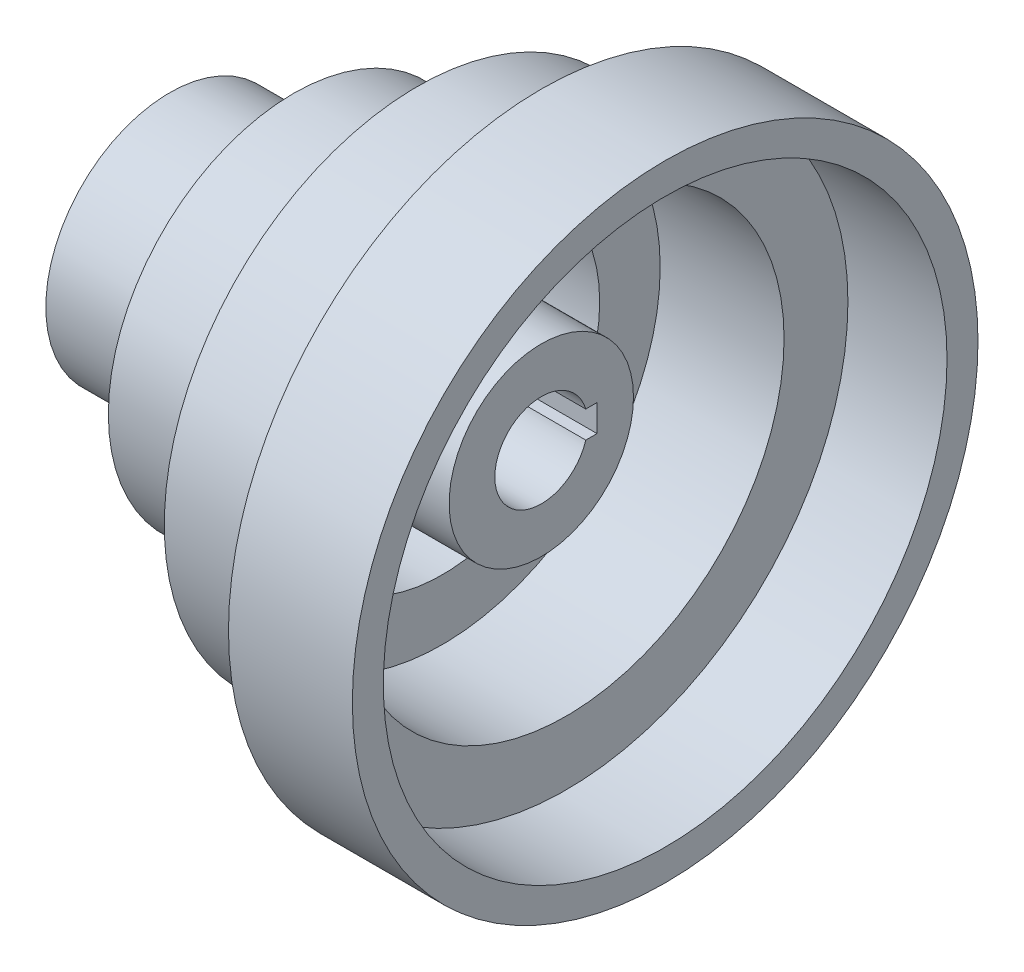
ISO-10303-21;
HEADER;
FILE_DESCRIPTION(('STEP AP214'),'2;1');
FILE_NAME('part.step','',(''),(''),'','','');
FILE_SCHEMA(('AUTOMOTIVE_DESIGN { 1 0 10303 214 1 1 1 1 }'));
ENDSEC;
DATA;
#1=APPLICATION_CONTEXT('core data for automotive mechanical design processes');
#2=APPLICATION_PROTOCOL_DEFINITION('international standard','automotive_design',2000,#1);
#3=PRODUCT_CONTEXT('',#1,'mechanical');
#4=PRODUCT('Part','Part','',(#3));
#5=PRODUCT_RELATED_PRODUCT_CATEGORY('part','',(#4));
#6=PRODUCT_DEFINITION_FORMATION('','',#4);
#7=PRODUCT_DEFINITION_CONTEXT('part definition',#1,'design');
#8=PRODUCT_DEFINITION('design','',#6,#7);
#9=PRODUCT_DEFINITION_SHAPE('','',#8);
#10=(LENGTH_UNIT() NAMED_UNIT(*) SI_UNIT(.MILLI.,.METRE.));
#11=(NAMED_UNIT(*) PLANE_ANGLE_UNIT() SI_UNIT($,.RADIAN.));
#12=(NAMED_UNIT(*) SI_UNIT($,.STERADIAN.) SOLID_ANGLE_UNIT());
#13=UNCERTAINTY_MEASURE_WITH_UNIT(LENGTH_MEASURE(1.E-05),#10,'distance_accuracy_value','');
#14=(GEOMETRIC_REPRESENTATION_CONTEXT(3) GLOBAL_UNCERTAINTY_ASSIGNED_CONTEXT((#13)) GLOBAL_UNIT_ASSIGNED_CONTEXT((#10,
#11,#12)) REPRESENTATION_CONTEXT('',''));
#15=CARTESIAN_POINT('',(0.,0.,0.));
#16=DIRECTION('',(0.,0.,1.));
#17=DIRECTION('',(1.,0.,0.));
#18=AXIS2_PLACEMENT_3D('',#15,#16,#17);
#19=CARTESIAN_POINT('',(151.689826596154,0.,0.));
#20=DIRECTION('',(1.,0.,0.));
#21=DIRECTION('',(0.,0.,-1.));
#22=AXIS2_PLACEMENT_3D('',#19,#20,#21);
#23=CYLINDRICAL_SURFACE('',#22,15.);
#24=DIRECTION('',(1.,0.,0.));
#25=VECTOR('',#24,1.);
#26=CARTESIAN_POINT('',(151.689826596154,4.34007504449317,-14.3584034143134));
#27=LINE('',#26,#25);
#28=CARTESIAN_POINT('',(64.9299911946379,4.34007504449317,-14.3584034143134));
#29=VERTEX_POINT('',#28);
#30=CARTESIAN_POINT('',(-55.0700088053621,4.34007504449317,-14.3584034143134));
#31=VERTEX_POINT('',#30);
#32=EDGE_CURVE('E58',#29,#31,#27,.F.);
#33=ORIENTED_EDGE('',*,*,#32,.F.);
#34=CARTESIAN_POINT('',(64.9299911946379,0.,0.));
#35=DIRECTION('',(1.,0.,0.));
#36=DIRECTION('',(0.,0.,-1.));
#37=AXIS2_PLACEMENT_3D('',#34,#35,#36);
#38=CIRCLE('',#37,15.);
#39=CARTESIAN_POINT('',(64.9299911946379,-4.34007504449317,-14.3584034143134));
#40=VERTEX_POINT('',#39);
#41=EDGE_CURVE('E102',#29,#40,#38,.T.);
#42=ORIENTED_EDGE('',*,*,#41,.T.);
#43=DIRECTION('',(1.,0.,0.));
#44=VECTOR('',#43,1.);
#45=CARTESIAN_POINT('',(151.689826596154,-4.34007504449317,-14.3584034143134));
#46=LINE('',#45,#44);
#47=CARTESIAN_POINT('',(-55.0700088053621,-4.34007504449317,-14.3584034143134));
#48=VERTEX_POINT('',#47);
#49=EDGE_CURVE('E52',#48,#40,#46,.T.);
#50=ORIENTED_EDGE('',*,*,#49,.F.);
#51=CARTESIAN_POINT('',(-55.0700088053621,0.,0.));
#52=DIRECTION('',(1.,0.,0.));
#53=DIRECTION('',(0.,0.,-1.));
#54=AXIS2_PLACEMENT_3D('',#51,#52,#53);
#55=CIRCLE('',#54,15.);
#56=EDGE_CURVE('E100',#31,#48,#55,.T.);
#57=ORIENTED_EDGE('',*,*,#56,.F.);
#58=EDGE_LOOP('',(#33,#42,#50,#57));
#59=FACE_BOUND('',#58,.T.);
#60=ADVANCED_FACE('F39',(#59),#23,.F.);
#61=CARTESIAN_POINT('',(-55.0700088053621,15.,0.));
#62=DIRECTION('',(-1.,0.,0.));
#63=DIRECTION('',(0.,0.,1.));
#64=AXIS2_PLACEMENT_3D('',#61,#62,#63);
#65=PLANE('',#64);
#66=DIRECTION('',(0.,0.,-1.));
#67=VECTOR('',#66,1.);
#68=CARTESIAN_POINT('',(-55.0700088053621,4.34007504449317,0.));
#69=LINE('',#68,#67);
#70=CARTESIAN_POINT('',(-55.0700088053621,4.34007504449317,-18.));
#71=VERTEX_POINT('',#70);
#72=EDGE_CURVE('E105',#31,#71,#69,.T.);
#73=ORIENTED_EDGE('',*,*,#72,.F.);
#74=ORIENTED_EDGE('',*,*,#56,.T.);
#75=DIRECTION('',(0.,0.,1.));
#76=VECTOR('',#75,1.);
#77=CARTESIAN_POINT('',(-55.0700088053621,-4.34007504449317,0.));
#78=LINE('',#77,#76);
#79=CARTESIAN_POINT('',(-55.0700088053621,-4.34007504449317,-18.));
#80=VERTEX_POINT('',#79);
#81=EDGE_CURVE('E86',#80,#48,#78,.T.);
#82=ORIENTED_EDGE('',*,*,#81,.F.);
#83=DIRECTION('',(0.,-1.,0.));
#84=VECTOR('',#83,1.);
#85=CARTESIAN_POINT('',(-55.0700088053621,15.,-18.));
#86=LINE('',#85,#84);
#87=EDGE_CURVE('E76',#71,#80,#86,.T.);
#88=ORIENTED_EDGE('',*,*,#87,.F.);
#89=EDGE_LOOP('',(#73,#74,#82,#88));
#90=FACE_BOUND('',#89,.T.);
#91=CARTESIAN_POINT('',(-55.0700088053621,0.,0.));
#92=DIRECTION('',(1.,0.,0.));
#93=DIRECTION('',(0.,0.,-1.));
#94=AXIS2_PLACEMENT_3D('',#91,#92,#93);
#95=CIRCLE('',#94,40.);
#96=CARTESIAN_POINT('',(-55.0700088053621,0.,-40.));
#97=VERTEX_POINT('',#96);
#98=EDGE_CURVE('E155',#97,#97,#95,.T.);
#99=ORIENTED_EDGE('',*,*,#98,.F.);
#100=EDGE_LOOP('',(#99));
#101=FACE_BOUND('',#100,.T.);
#102=ADVANCED_FACE('F94',(#90,#101),#65,.T.);
#103=CARTESIAN_POINT('',(151.689826596154,0.,0.));
#104=DIRECTION('',(1.,0.,0.));
#105=DIRECTION('',(0.,0.,-1.));
#106=AXIS2_PLACEMENT_3D('',#103,#104,#105);
#107=CYLINDRICAL_SURFACE('',#106,40.);
#108=ORIENTED_EDGE('',*,*,#98,.T.);
#109=EDGE_LOOP('',(#108));
#110=FACE_BOUND('',#109,.T.);
#111=CARTESIAN_POINT('',(-15.0700088053621,0.,0.));
#112=DIRECTION('',(1.,0.,0.));
#113=DIRECTION('',(0.,0.,-1.));
#114=AXIS2_PLACEMENT_3D('',#111,#112,#113);
#115=CIRCLE('',#114,40.);
#116=CARTESIAN_POINT('',(-15.0700088053621,0.,-40.));
#117=VERTEX_POINT('',#116);
#118=EDGE_CURVE('E149',#117,#117,#115,.T.);
#119=ORIENTED_EDGE('',*,*,#118,.F.);
#120=EDGE_LOOP('',(#119));
#121=FACE_BOUND('',#120,.T.);
#122=ADVANCED_FACE('F166',(#110,#121),#107,.T.);
#123=CARTESIAN_POINT('',(-15.0700088053621,40.,0.));
#124=DIRECTION('',(-1.,0.,0.));
#125=DIRECTION('',(0.,0.,1.));
#126=AXIS2_PLACEMENT_3D('',#123,#124,#125);
#127=PLANE('',#126);
#128=ORIENTED_EDGE('',*,*,#118,.T.);
#129=EDGE_LOOP('',(#128));
#130=FACE_BOUND('',#129,.T.);
#131=CARTESIAN_POINT('',(-15.0700088053621,0.,0.));
#132=DIRECTION('',(1.,0.,0.));
#133=DIRECTION('',(0.,0.,-1.));
#134=AXIS2_PLACEMENT_3D('',#131,#132,#133);
#135=CIRCLE('',#134,59.802619068126);
#136=CARTESIAN_POINT('',(-15.0700088053621,0.,-59.802619068126));
#137=VERTEX_POINT('',#136);
#138=EDGE_CURVE('E148',#137,#137,#135,.T.);
#139=ORIENTED_EDGE('',*,*,#138,.F.);
#140=EDGE_LOOP('',(#139));
#141=FACE_BOUND('',#140,.T.);
#142=ADVANCED_FACE('F171',(#130,#141),#127,.T.);
#143=CARTESIAN_POINT('',(151.689826596154,0.,0.));
#144=DIRECTION('',(1.,0.,0.));
#145=DIRECTION('',(0.,0.,-1.));
#146=AXIS2_PLACEMENT_3D('',#143,#144,#145);
#147=CYLINDRICAL_SURFACE('',#146,59.802619068126);
#148=ORIENTED_EDGE('',*,*,#138,.T.);
#149=EDGE_LOOP('',(#148));
#150=FACE_BOUND('',#149,.T.);
#151=CARTESIAN_POINT('',(24.9299911946379,0.,0.));
#152=DIRECTION('',(1.,0.,0.));
#153=DIRECTION('',(0.,0.,-1.));
#154=AXIS2_PLACEMENT_3D('',#151,#152,#153);
#155=CIRCLE('',#154,59.802619068126);
#156=CARTESIAN_POINT('',(24.9299911946379,0.,-59.802619068126));
#157=VERTEX_POINT('',#156);
#158=EDGE_CURVE('E141',#157,#157,#155,.T.);
#159=ORIENTED_EDGE('',*,*,#158,.F.);
#160=EDGE_LOOP('',(#159));
#161=FACE_BOUND('',#160,.T.);
#162=ADVANCED_FACE('F179',(#150,#161),#147,.T.);
#163=CARTESIAN_POINT('',(24.9299911946379,59.802619068126,0.));
#164=DIRECTION('',(-1.,0.,0.));
#165=DIRECTION('',(0.,0.,1.));
#166=AXIS2_PLACEMENT_3D('',#163,#164,#165);
#167=PLANE('',#166);
#168=ORIENTED_EDGE('',*,*,#158,.T.);
#169=EDGE_LOOP('',(#168));
#170=FACE_BOUND('',#169,.T.);
#171=CARTESIAN_POINT('',(24.9299911946379,0.,0.));
#172=DIRECTION('',(1.,0.,0.));
#173=DIRECTION('',(0.,0.,-1.));
#174=AXIS2_PLACEMENT_3D('',#171,#172,#173);
#175=CIRCLE('',#174,81.7460618192928);
#176=CARTESIAN_POINT('',(24.9299911946379,0.,-81.7460618192928));
#177=VERTEX_POINT('',#176);
#178=EDGE_CURVE('E139',#177,#177,#175,.T.);
#179=ORIENTED_EDGE('',*,*,#178,.F.);
#180=EDGE_LOOP('',(#179));
#181=FACE_BOUND('',#180,.T.);
#182=ADVANCED_FACE('F184',(#170,#181),#167,.T.);
#183=CARTESIAN_POINT('',(151.689826596154,0.,0.));
#184=DIRECTION('',(1.,0.,0.));
#185=DIRECTION('',(0.,0.,-1.));
#186=AXIS2_PLACEMENT_3D('',#183,#184,#185);
#187=CYLINDRICAL_SURFACE('',#186,81.7460618192928);
#188=ORIENTED_EDGE('',*,*,#178,.T.);
#189=EDGE_LOOP('',(#188));
#190=FACE_BOUND('',#189,.T.);
#191=CARTESIAN_POINT('',(64.9299911946379,0.,0.));
#192=DIRECTION('',(1.,0.,0.));
#193=DIRECTION('',(0.,0.,-1.));
#194=AXIS2_PLACEMENT_3D('',#191,#192,#193);
#195=CIRCLE('',#194,81.7460618192928);
#196=CARTESIAN_POINT('',(64.9299911946379,0.,-81.7460618192928));
#197=VERTEX_POINT('',#196);
#198=EDGE_CURVE('E140',#197,#197,#195,.T.);
#199=ORIENTED_EDGE('',*,*,#198,.F.);
#200=EDGE_LOOP('',(#199));
#201=FACE_BOUND('',#200,.T.);
#202=ADVANCED_FACE('F189',(#190,#201),#187,.T.);
#203=CARTESIAN_POINT('',(64.9299911946379,81.7460618192928,0.));
#204=DIRECTION('',(-1.,0.,0.));
#205=DIRECTION('',(0.,0.,1.));
#206=AXIS2_PLACEMENT_3D('',#203,#204,#205);
#207=PLANE('',#206);
#208=ORIENTED_EDGE('',*,*,#198,.T.);
#209=EDGE_LOOP('',(#208));
#210=FACE_BOUND('',#209,.T.);
#211=CARTESIAN_POINT('',(64.9299911946379,0.,0.));
#212=DIRECTION('',(1.,0.,0.));
#213=DIRECTION('',(0.,0.,-1.));
#214=AXIS2_PLACEMENT_3D('',#211,#212,#213);
#215=CIRCLE('',#214,101.013474966659);
#216=CARTESIAN_POINT('',(64.9299911946379,0.,-101.013474966659));
#217=VERTEX_POINT('',#216);
#218=EDGE_CURVE('E131',#217,#217,#215,.T.);
#219=ORIENTED_EDGE('',*,*,#218,.F.);
#220=EDGE_LOOP('',(#219));
#221=FACE_BOUND('',#220,.T.);
#222=ADVANCED_FACE('F195',(#210,#221),#207,.T.);
#223=CARTESIAN_POINT('',(151.689826596154,0.,0.));
#224=DIRECTION('',(1.,0.,0.));
#225=DIRECTION('',(0.,0.,-1.));
#226=AXIS2_PLACEMENT_3D('',#223,#224,#225);
#227=CYLINDRICAL_SURFACE('',#226,101.013474966659);
#228=ORIENTED_EDGE('',*,*,#218,.T.);
#229=EDGE_LOOP('',(#228));
#230=FACE_BOUND('',#229,.T.);
#231=CARTESIAN_POINT('',(104.929991194638,0.,0.));
#232=DIRECTION('',(1.,0.,0.));
#233=DIRECTION('',(0.,0.,-1.));
#234=AXIS2_PLACEMENT_3D('',#231,#232,#233);
#235=CIRCLE('',#234,101.013474966659);
#236=CARTESIAN_POINT('',(104.929991194638,0.,-101.013474966659));
#237=VERTEX_POINT('',#236);
#238=EDGE_CURVE('E132',#237,#237,#235,.T.);
#239=ORIENTED_EDGE('',*,*,#238,.F.);
#240=EDGE_LOOP('',(#239));
#241=FACE_BOUND('',#240,.T.);
#242=ADVANCED_FACE('F198',(#230,#241),#227,.T.);
#243=CARTESIAN_POINT('',(104.929991194638,101.013474966659,0.));
#244=DIRECTION('',(1.,0.,0.));
#245=DIRECTION('',(0.,0.,-1.));
#246=AXIS2_PLACEMENT_3D('',#243,#244,#245);
#247=PLANE('',#246);
#248=ORIENTED_EDGE('',*,*,#238,.T.);
#249=EDGE_LOOP('',(#248));
#250=FACE_BOUND('',#249,.T.);
#251=CARTESIAN_POINT('',(104.929991194638,0.,0.));
#252=DIRECTION('',(1.,0.,0.));
#253=DIRECTION('',(0.,0.,-1.));
#254=AXIS2_PLACEMENT_3D('',#251,#252,#253);
#255=CIRCLE('',#254,91.0134749666587);
#256=CARTESIAN_POINT('',(104.929991194638,0.,-91.0134749666587));
#257=VERTEX_POINT('',#256);
#258=EDGE_CURVE('E126',#257,#257,#255,.T.);
#259=ORIENTED_EDGE('',*,*,#258,.F.);
#260=EDGE_LOOP('',(#259));
#261=FACE_BOUND('',#260,.T.);
#262=ADVANCED_FACE('F199',(#250,#261),#247,.T.);
#263=CARTESIAN_POINT('',(151.689826596154,0.,0.));
#264=DIRECTION('',(1.,0.,0.));
#265=DIRECTION('',(0.,0.,-1.));
#266=AXIS2_PLACEMENT_3D('',#263,#264,#265);
#267=CYLINDRICAL_SURFACE('',#266,91.0134749666587);
#268=ORIENTED_EDGE('',*,*,#258,.T.);
#269=EDGE_LOOP('',(#268));
#270=FACE_BOUND('',#269,.T.);
#271=CARTESIAN_POINT('',(72.9299911946379,0.,0.));
#272=DIRECTION('',(1.,0.,0.));
#273=DIRECTION('',(0.,0.,-1.));
#274=AXIS2_PLACEMENT_3D('',#271,#272,#273);
#275=CIRCLE('',#274,91.0134749666587);
#276=CARTESIAN_POINT('',(72.9299911946379,0.,-91.0134749666587));
#277=VERTEX_POINT('',#276);
#278=EDGE_CURVE('E124',#277,#277,#275,.T.);
#279=ORIENTED_EDGE('',*,*,#278,.F.);
#280=EDGE_LOOP('',(#279));
#281=FACE_BOUND('',#280,.T.);
#282=ADVANCED_FACE('F204',(#270,#281),#267,.F.);
#283=CARTESIAN_POINT('',(72.9299911946379,91.0134749666587,0.));
#284=DIRECTION('',(1.,0.,0.));
#285=DIRECTION('',(0.,0.,-1.));
#286=AXIS2_PLACEMENT_3D('',#283,#284,#285);
#287=PLANE('',#286);
#288=ORIENTED_EDGE('',*,*,#278,.T.);
#289=EDGE_LOOP('',(#288));
#290=FACE_BOUND('',#289,.T.);
#291=CARTESIAN_POINT('',(72.9299911946379,0.,0.));
#292=DIRECTION('',(1.,0.,0.));
#293=DIRECTION('',(0.,0.,-1.));
#294=AXIS2_PLACEMENT_3D('',#291,#292,#293);
#295=CIRCLE('',#294,70.3938127986771);
#296=CARTESIAN_POINT('',(72.9299911946379,0.,-70.3938127986771));
#297=VERTEX_POINT('',#296);
#298=EDGE_CURVE('E125',#297,#297,#295,.T.);
#299=ORIENTED_EDGE('',*,*,#298,.F.);
#300=EDGE_LOOP('',(#299));
#301=FACE_BOUND('',#300,.T.);
#302=ADVANCED_FACE('F208',(#290,#301),#287,.T.);
#303=CARTESIAN_POINT('',(151.689826596154,0.,0.));
#304=DIRECTION('',(1.,0.,0.));
#305=DIRECTION('',(0.,0.,-1.));
#306=AXIS2_PLACEMENT_3D('',#303,#304,#305);
#307=CYLINDRICAL_SURFACE('',#306,70.3938127986771);
#308=ORIENTED_EDGE('',*,*,#298,.T.);
#309=EDGE_LOOP('',(#308));
#310=FACE_BOUND('',#309,.T.);
#311=CARTESIAN_POINT('',(32.9299911946379,0.,0.));
#312=DIRECTION('',(1.,0.,0.));
#313=DIRECTION('',(0.,0.,-1.));
#314=AXIS2_PLACEMENT_3D('',#311,#312,#313);
#315=CIRCLE('',#314,70.3938127986771);
#316=CARTESIAN_POINT('',(32.9299911946379,0.,-70.3938127986771));
#317=VERTEX_POINT('',#316);
#318=EDGE_CURVE('E116',#317,#317,#315,.T.);
#319=ORIENTED_EDGE('',*,*,#318,.F.);
#320=EDGE_LOOP('',(#319));
#321=FACE_BOUND('',#320,.T.);
#322=ADVANCED_FACE('F215',(#310,#321),#307,.F.);
#323=CARTESIAN_POINT('',(32.9299911946379,70.3938127986771,0.));
#324=DIRECTION('',(1.,0.,0.));
#325=DIRECTION('',(0.,0.,-1.));
#326=AXIS2_PLACEMENT_3D('',#323,#324,#325);
#327=PLANE('',#326);
#328=ORIENTED_EDGE('',*,*,#318,.T.);
#329=EDGE_LOOP('',(#328));
#330=FACE_BOUND('',#329,.T.);
#331=CARTESIAN_POINT('',(32.9299911946379,0.,0.));
#332=DIRECTION('',(1.,0.,0.));
#333=DIRECTION('',(0.,0.,-1.));
#334=AXIS2_PLACEMENT_3D('',#331,#332,#333);
#335=CIRCLE('',#334,50.8587966909311);
#336=CARTESIAN_POINT('',(32.9299911946379,0.,-50.8587966909311));
#337=VERTEX_POINT('',#336);
#338=EDGE_CURVE('E117',#337,#337,#335,.T.);
#339=ORIENTED_EDGE('',*,*,#338,.F.);
#340=EDGE_LOOP('',(#339));
#341=FACE_BOUND('',#340,.T.);
#342=ADVANCED_FACE('F216',(#330,#341),#327,.T.);
#343=CARTESIAN_POINT('',(151.689826596154,0.,0.));
#344=DIRECTION('',(1.,0.,0.));
#345=DIRECTION('',(0.,0.,-1.));
#346=AXIS2_PLACEMENT_3D('',#343,#344,#345);
#347=CYLINDRICAL_SURFACE('',#346,50.8587966909311);
#348=ORIENTED_EDGE('',*,*,#338,.T.);
#349=EDGE_LOOP('',(#348));
#350=FACE_BOUND('',#349,.T.);
#351=CARTESIAN_POINT('',(-7.0700088053621,0.,0.));
#352=DIRECTION('',(1.,0.,0.));
#353=DIRECTION('',(0.,0.,-1.));
#354=AXIS2_PLACEMENT_3D('',#351,#352,#353);
#355=CIRCLE('',#354,50.8587966909311);
#356=CARTESIAN_POINT('',(-7.0700088053621,0.,-50.8587966909311));
#357=VERTEX_POINT('',#356);
#358=EDGE_CURVE('E114',#357,#357,#355,.T.);
#359=ORIENTED_EDGE('',*,*,#358,.F.);
#360=EDGE_LOOP('',(#359));
#361=FACE_BOUND('',#360,.T.);
#362=ADVANCED_FACE('F219',(#350,#361),#347,.F.);
#363=CARTESIAN_POINT('',(-7.07000880536211,50.8587966909311,0.));
#364=DIRECTION('',(1.,0.,0.));
#365=DIRECTION('',(0.,0.,-1.));
#366=AXIS2_PLACEMENT_3D('',#363,#364,#365);
#367=PLANE('',#366);
#368=ORIENTED_EDGE('',*,*,#358,.T.);
#369=EDGE_LOOP('',(#368));
#370=FACE_BOUND('',#369,.T.);
#371=CARTESIAN_POINT('',(-7.0700088053621,0.,0.));
#372=DIRECTION('',(1.,0.,0.));
#373=DIRECTION('',(0.,0.,-1.));
#374=AXIS2_PLACEMENT_3D('',#371,#372,#373);
#375=CIRCLE('',#374,29.7651458726585);
#376=CARTESIAN_POINT('',(-7.0700088053621,0.,-29.7651458726585));
#377=VERTEX_POINT('',#376);
#378=EDGE_CURVE('E109',#377,#377,#375,.T.);
#379=ORIENTED_EDGE('',*,*,#378,.F.);
#380=EDGE_LOOP('',(#379));
#381=FACE_BOUND('',#380,.T.);
#382=ADVANCED_FACE('F221',(#370,#381),#367,.T.);
#383=CARTESIAN_POINT('',(151.689826596154,0.,0.));
#384=DIRECTION('',(1.,0.,0.));
#385=DIRECTION('',(0.,0.,-1.));
#386=AXIS2_PLACEMENT_3D('',#383,#384,#385);
#387=CYLINDRICAL_SURFACE('',#386,29.7651458726585);
#388=ORIENTED_EDGE('',*,*,#378,.T.);
#389=EDGE_LOOP('',(#388));
#390=FACE_BOUND('',#389,.T.);
#391=CARTESIAN_POINT('',(64.9299911946379,0.,0.));
#392=DIRECTION('',(1.,0.,0.));
#393=DIRECTION('',(0.,0.,-1.));
#394=AXIS2_PLACEMENT_3D('',#391,#392,#393);
#395=CIRCLE('',#394,29.7651458726585);
#396=CARTESIAN_POINT('',(64.9299911946379,0.,-29.7651458726585));
#397=VERTEX_POINT('',#396);
#398=EDGE_CURVE('E110',#397,#397,#395,.T.);
#399=ORIENTED_EDGE('',*,*,#398,.F.);
#400=EDGE_LOOP('',(#399));
#401=FACE_BOUND('',#400,.T.);
#402=ADVANCED_FACE('F229',(#390,#401),#387,.T.);
#403=CARTESIAN_POINT('',(64.9299911946379,29.7651458726585,0.));
#404=DIRECTION('',(1.,0.,0.));
#405=DIRECTION('',(0.,0.,-1.));
#406=AXIS2_PLACEMENT_3D('',#403,#404,#405);
#407=PLANE('',#406);
#408=DIRECTION('',(0.,0.,1.));
#409=VECTOR('',#408,1.);
#410=CARTESIAN_POINT('',(64.9299911946379,4.34007504449317,0.));
#411=LINE('',#410,#409);
#412=CARTESIAN_POINT('',(64.9299911946379,4.34007504449317,-18.));
#413=VERTEX_POINT('',#412);
#414=EDGE_CURVE('E11',#413,#29,#411,.T.);
#415=ORIENTED_EDGE('',*,*,#414,.F.);
#416=DIRECTION('',(0.,1.,0.));
#417=VECTOR('',#416,1.);
#418=CARTESIAN_POINT('',(64.9299911946379,29.7651458726585,-18.));
#419=LINE('',#418,#417);
#420=CARTESIAN_POINT('',(64.9299911946379,-4.34007504449317,-18.));
#421=VERTEX_POINT('',#420);
#422=EDGE_CURVE('E46',#421,#413,#419,.T.);
#423=ORIENTED_EDGE('',*,*,#422,.F.);
#424=DIRECTION('',(0.,0.,-1.));
#425=VECTOR('',#424,1.);
#426=CARTESIAN_POINT('',(64.9299911946379,-4.34007504449317,0.));
#427=LINE('',#426,#425);
#428=EDGE_CURVE('E93',#40,#421,#427,.T.);
#429=ORIENTED_EDGE('',*,*,#428,.F.);
#430=ORIENTED_EDGE('',*,*,#41,.F.);
#431=EDGE_LOOP('',(#415,#423,#429,#430));
#432=FACE_BOUND('',#431,.T.);
#433=ORIENTED_EDGE('',*,*,#398,.T.);
#434=EDGE_LOOP('',(#433));
#435=FACE_BOUND('',#434,.T.);
#436=ADVANCED_FACE('F161',(#432,#435),#407,.T.);
#437=CARTESIAN_POINT('',(-110.,4.34007504449317,-3.));
#438=DIRECTION('',(0.,1.,0.));
#439=DIRECTION('',(0.,0.,1.));
#440=AXIS2_PLACEMENT_3D('',#437,#438,#439);
#441=PLANE('',#440);
#442=ORIENTED_EDGE('',*,*,#72,.T.);
#443=DIRECTION('',(1.,0.,0.));
#444=VECTOR('',#443,1.);
#445=CARTESIAN_POINT('',(-110.,4.34007504449317,-18.));
#446=LINE('',#445,#444);
#447=EDGE_CURVE('E84',#71,#413,#446,.T.);
#448=ORIENTED_EDGE('',*,*,#447,.T.);
#449=ORIENTED_EDGE('',*,*,#414,.T.);
#450=ORIENTED_EDGE('',*,*,#32,.T.);
#451=EDGE_LOOP('',(#442,#448,#449,#450));
#452=FACE_BOUND('',#451,.T.);
#453=ADVANCED_FACE('F158',(#452),#441,.F.);
#454=CARTESIAN_POINT('',(-110.,4.34007504449317,-18.));
#455=DIRECTION('',(0.,0.,-1.));
#456=DIRECTION('',(-1.,0.,0.));
#457=AXIS2_PLACEMENT_3D('',#454,#455,#456);
#458=PLANE('',#457);
#459=ORIENTED_EDGE('',*,*,#87,.T.);
#460=DIRECTION('',(1.,0.,0.));
#461=VECTOR('',#460,1.);
#462=CARTESIAN_POINT('',(-110.,-4.34007504449317,-18.));
#463=LINE('',#462,#461);
#464=EDGE_CURVE('E85',#80,#421,#463,.T.);
#465=ORIENTED_EDGE('',*,*,#464,.T.);
#466=ORIENTED_EDGE('',*,*,#422,.T.);
#467=ORIENTED_EDGE('',*,*,#447,.F.);
#468=EDGE_LOOP('',(#459,#465,#466,#467));
#469=FACE_BOUND('',#468,.T.);
#470=ADVANCED_FACE('F83',(#469),#458,.F.);
#471=CARTESIAN_POINT('',(-110.,-4.34007504449317,-3.));
#472=DIRECTION('',(0.,-1.,0.));
#473=DIRECTION('',(0.,0.,-1.));
#474=AXIS2_PLACEMENT_3D('',#471,#472,#473);
#475=PLANE('',#474);
#476=ORIENTED_EDGE('',*,*,#81,.T.);
#477=ORIENTED_EDGE('',*,*,#49,.T.);
#478=ORIENTED_EDGE('',*,*,#428,.T.);
#479=ORIENTED_EDGE('',*,*,#464,.F.);
#480=EDGE_LOOP('',(#476,#477,#478,#479));
#481=FACE_BOUND('',#480,.T.);
#482=ADVANCED_FACE('F89',(#481),#475,.F.);
#483=CLOSED_SHELL('',(#60,#102,#122,#142,#162,#182,#202,#222,#242,#262,#282,#302,#322,#342,#362,
#382,#402,#436,#453,#470,#482));
#484=MANIFOLD_SOLID_BREP('B2',#483);
#485=ADVANCED_BREP_SHAPE_REPRESENTATION('',(#18,#484),#14);
#486=SHAPE_DEFINITION_REPRESENTATION(#9,#485);
ENDSEC;
END-ISO-10303-21;
